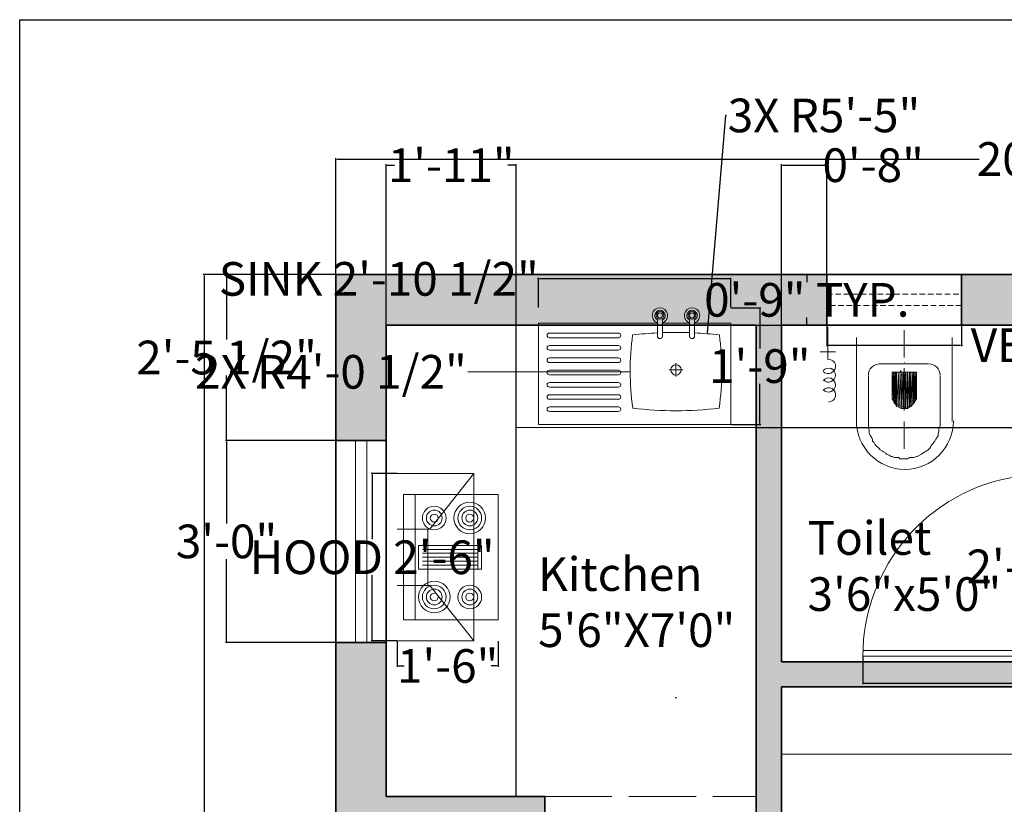
# Model space of a CAD drawing. Units: inches. Extents: x 335 to 688, y 1043 to 1486.
# Tile 4 of 7: x 335 to 510, y 1347 to 1486. Entities that reach past the tile are written whole.
import ezdxf

# ---------------------------------------------------------------- set-up
doc = ezdxf.new("R2010")
doc.units = ezdxf.units.IN
doc.header["$MEASUREMENT"] = 0
doc.linetypes.add('ACAD_ISO02W100', pattern=[15, 12, -3])
doc.linetypes.add('DASHEDX2', pattern=[1.5, 1, -0.5])
for name, color, linetype, lineweight in [('A-ANNO-DIMS', 2, 'Continuous', 18), ('A-ANNO-TTLB', 7, 'Continuous', 25), ('A-AREA-IDEN', 7, 'Continuous', 18), ('A-DOOR', 4, 'Continuous', 18), ('A-EQPM', 8, 'Continuous', 18), ('A-FLOR-CASE', 8, 'Continuous', 18), ('A-FLOR-FIXT', 8, 'Continuous', 18), ('A-GLAZ', 4, 'Continuous', 18), ('A-GLAZ-VENT', 4, 'DASHEDX2', 18), ('A-WALL', 7, 'Continuous', 35), ('A-WALL-OVHD', 7, 'ACAD_ISO02W100', 18), ('A-WALL-PATT', 252, 'Continuous', 13)]:
    doc.layers.add(name, color=color, linetype=linetype, lineweight=lineweight)
doc.styles.get("Standard").update_dxf_attribs({"font": 'arial.ttf'})
doc.dimstyles.get("Standard").update_dxf_attribs({"dimtxt": 6, "dimasz": 0.18, "dimexe": 0.18, "dimexo": 0.0625, "dimgap": 0.09, "dimtad": 0, "dimtih": 1, "dimtoh": 1, "dimdec": 1, "dimzin": 0, "dimdsep": 46, "dimlunit": 3, "dimtxsty": 'Standard', "dimcen": 0.09, "dimadec": 0, "dimazin": 0, "dimtfac": 1, "dimtdec": 1, "dimtofl": 0, "dimtmove": 0, "dimatfit": 3, "dimfxl": 1, "dimtolj": 1, "dimtzin": 0, "dimarcsym": 0})

# ---------------------------------------------------------------- blocks, each defined once
blk = doc.blocks.new('chimmne')
for p, q in [((17.89, 6.07), (-18.11, 6.07)), ((-18.11, 6.07), (-18.11, -10.43)), ((-6.16, -3.43), (-18.11, 6.07)), ((5.94, -3.43), (17.89, 6.07)), ((17.89, 6.07), (17.89, -10.43)), ((-6.16, -3.43), (-6.16, -10.43)), ((5.94, -3.82), (-6.16, -3.82)), ((5.94, -3.43), (5.94, -10.43))]:
    blk.add_line(p, q)
for points in [[(-13.61, -9.12), (-13.61, 11.28), (13.39, 11.28), (13.39, -9.12)], [(-2.66, -5.87), (-2.66, 7.73), (2.44, 7.73), (2.44, -5.87)]]:
    blk.add_lwpolyline(points, close=True)
for points in [[(-2.66, 6.88), (2.44, 6.88)], [(-1.81, 6.88), (-1.81, -5.02)], [(-0.96, -5.02), (-0.96, 6.88)], [(-0.11, 6.88), (-0.11, -5.02)], [(0.74, -5.02), (0.74, 6.88)], [(1.59, 6.88), (1.59, -5.02)], [(13.39, -6.57), (-13.61, -6.57)]]:
    blk.add_lwpolyline(points)
for centre, radius in [((-8.55, 5.18), 3.4), ((-8.55, 5.18), 2.55), ((-8.55, 5.18), 1.7), ((8.44, 5.18), 2.55), ((8.44, 5.18), 1.7), ((-8.55, 5.18), 0.85), ((8.44, 5.18), 0.85), ((-8.55, -2.47), 2.55), ((8.44, -2.47), 3.4), ((8.44, -2.47), 2.55), ((-8.55, -2.47), 1.7), ((-8.55, -2.47), 0.85), ((8.44, -2.47), 1.7), ((8.44, -2.47), 0.85)]:
    blk.add_circle(centre, radius)
blk = doc.blocks.new('A$C799204C7')
for p, q in [((0, 34.2), (17.99, 34.2)), ((0, 0), (0, 34.2)), ((17.99, 13.08), (17.99, 34.2)), ((2.32, 20.01), (2.32, 32.27)), ((3.13, 20.01), (3.13, 32.27)), ((4.48, 20.01), (4.48, 32.27)), ((5.29, 20.01), (5.29, 32.27)), ((6.64, 20.01), (6.64, 32.27)), ((7.45, 20.01), (7.45, 32.27)), ((8.85, 20.01), (8.85, 32.27)), ((9.66, 20.01), (9.66, 32.27)), ((11.01, 20.01), (11.01, 32.27)), ((11.82, 20.01), (11.82, 32.27)), ((13.22, 20.01), (13.22, 32.27)), ((14.03, 20.01), (14.03, 32.27)), ((15.42, 20.01), (15.42, 32.27)), ((16.24, 20.01), (16.24, 32.27)), ((18.59, 13.08), (15.71, 13.08)), ((9.73, 11), (9.73, 8.54)), ((15.71, 12.17), (18.59, 12.17)), ((17.99, 7.36), (17.99, 12.17)), ((8.52, 9.77), (10.9, 9.77)), ((18.59, 7.36), (15.71, 7.36)), ((15.71, 6.45), (18.59, 6.45)), ((17.99, 0), (17.99, 6.45)), ((0, 0), (17.99, 0))]:
    blk.add_line(p, q)
for centre, radius in [((19.38, 12.62), 0.684), ((19.38, 12.62), 0.456), ((9.7, 9.77), 0.916), ((19.38, 6.91), 0.684), ((19.38, 6.91), 0.456)]:
    blk.add_circle(centre, radius)
for centre, radius, start, end in [((2.72, 32.27), 0.407, 0, 180), ((4.88, 32.27), 0.407, 0, 180), ((7.05, 32.27), 0.407, 0, 180), ((9.25, 32.27), 0.407, 0, 180), ((11.42, 32.27), 0.407, 0, 180), ((13.62, 32.27), 0.407, 0, 180), ((15.83, 32.27), 0.407, 0, 180), ((2.72, 20.01), 0.407, 180, 0), ((4.88, 20.01), 0.407, 180, 0), ((7.05, 20.01), 0.407, 180, 0), ((9.25, 20.01), 0.407, 180, 0), ((11.42, 20.01), 0.407, 180, 0), ((13.62, 20.01), 0.407, 180, 0), ((15.83, 20.01), 0.407, 180, 0), ((9.53, -30.19), 48.1, 82.3437, 97.8966), ((67.33, 9.77), 64.88, 173.1952, 186.8048), ((-48.51, 9.77), 64.88, 2.9208, 6.8048), ((15.71, 12.62), 0.456, 90, 270), ((19.38, 12.62), 1.37, 199.6514, 160.3603), ((19.38, 12.62), 0.911, 210.3431, 149.7554), ((-48.51, 9.77), 64.88, 357.8723, 2.115), ((15.71, 6.91), 0.456, 90, 270), ((19.38, 6.91), 1.37, 199.6514, 160.3603), ((19.38, 6.91), 0.911, 210.3431, 149.7554), ((-48.51, 9.77), 64.88, 353.1952, 357.0665), ((9.53, 49.73), 48.1, 262.1034, 277.6563)]:
    blk.add_arc(centre, radius, start, end)
blk = doc.blocks.new('*D3')
at = {"layer": 'A-ANNO-DIMS', "color": 0, "lineweight": -2, "transparency": 16777216}
for p, q in [((391.11, 1441.03), (391.11, 1461.75)), ((391.29, 1461.57), (505.87, 1461.57)), ((630.93, 1461.57), (516.34, 1461.57)), ((631.11, 1441.03), (631.11, 1461.75))]:
    blk.add_line(p, q, dxfattribs=at)
at = {"layer": 'A-ANNO-DIMS', "color": 0, "transparency": 16777216}
for points in [[(391.29, 1461.6), (391.29, 1461.54), (391.11, 1461.57)], [(630.93, 1461.6), (630.93, 1461.54), (631.11, 1461.57)]]:
    blk.add_solid(points, dxfattribs=at)
at = {"layer": 'Defpoints', "color": 0, "transparency": 16777216}
for p in [(631.11, 1461.57), (391.11, 1440.97), (631.11, 1440.97)]:
    blk.add_point(p, dxfattribs=at)
at = {"layer": 'A-ANNO-DIMS', "color": 0, "transparency": 16777216, "insert": (511.11, 1461.57), "char_height": 6, "attachment_point": 5}
blk.add_mtext("\\A1;20'", dxfattribs=at)
blk = doc.blocks.new('*D4')
at = {"layer": 'A-ANNO-DIMS', "color": 0, "lineweight": -2, "transparency": 16777216}
for p, q in [((391.04, 1440.97), (367.42, 1440.97)), ((367.6, 1440.79), (367.6, 1264.12)), ((367.6, 1081.15), (367.6, 1257.81)), ((391.04, 1080.97), (367.42, 1080.97))]:
    blk.add_line(p, q, dxfattribs=at)
at = {"layer": 'A-ANNO-DIMS', "color": 0, "transparency": 16777216}
for points in [[(367.57, 1440.79), (367.63, 1440.79), (367.6, 1440.97)], [(367.57, 1081.15), (367.63, 1081.15), (367.6, 1080.97)]]:
    blk.add_solid(points, dxfattribs=at)
at = {"layer": 'Defpoints', "color": 0, "transparency": 16777216}
for p in [(391.11, 1440.97), (367.6, 1080.97), (391.11, 1080.97)]:
    blk.add_point(p, dxfattribs=at)
at = {"layer": 'A-ANNO-DIMS', "color": 0, "transparency": 16777216, "insert": (367.6, 1260.97), "char_height": 6, "attachment_point": 5}
blk.add_mtext("\\A1;30'", dxfattribs=at)
blk = doc.blocks.new('WC')
h = blk.add_hatch(color=256)
h.paths.add_polyline_path([(17.3, 10.54), (11.83, 10.54), (17.3, 10.32)])
h.paths.add_polyline_path([(11.83, 10.54), (17.3, 10.32), (11.61, 10.32)])
h = blk.add_hatch(color=256)
h.paths.add_polyline_path([(17.3, 10.7), (12.21, 10.7), (17.3, 10.54)])
h.paths.add_polyline_path([(12.21, 10.7), (17.3, 10.54), (11.83, 10.54)])
h = blk.add_hatch(color=256)
h.paths.add_polyline_path([(17.3, 10.92), (12.59, 10.92), (17.3, 10.7)])
h.paths.add_polyline_path([(12.59, 10.92), (17.3, 10.7), (12.21, 10.7)])
h = blk.add_hatch(color=256)
h.paths.add_polyline_path([(17.3, 9.71), (11.08, 9.71), (17.3, 9.33)])
h.paths.add_polyline_path([(11.08, 9.71), (17.3, 9.33), (10.85, 9.33)])
h = blk.add_hatch(color=256)
h.paths.add_polyline_path([(17.3, 9.33), (10.85, 9.33), (17.3, 8.95)])
h.paths.add_polyline_path([(10.85, 9.33), (17.3, 8.95), (10.85, 8.95)])
h = blk.add_hatch(color=256)
h.paths.add_polyline_path([(17.3, 8.95), (10.85, 8.95), (17.3, 8.57)])
h.paths.add_polyline_path([(10.85, 8.95), (17.3, 8.57), (10.85, 8.57)])
h = blk.add_hatch(color=256)
h.paths.add_polyline_path([(17.3, 10.16), (11.23, 10.16), (17.3, 9.71)])
h.paths.add_polyline_path([(11.23, 10.16), (17.3, 9.71), (11.08, 9.71)])
h = blk.add_hatch(color=256)
h.paths.add_polyline_path([(17.3, 10.32), (11.61, 10.32), (17.3, 10.16)])
h.paths.add_polyline_path([(11.61, 10.32), (17.3, 10.16), (11.23, 10.16)])
h = blk.add_hatch(color=256)
h.paths.add_polyline_path([(17.3, 8.57), (10.85, 8.57), (17.3, 8.19)])
h.paths.add_polyline_path([(10.85, 8.57), (17.3, 8.19), (10.85, 8.19)])
h = blk.add_hatch(color=256)
h.paths.add_polyline_path([(17.3, 8.19), (10.85, 8.19), (17.3, 7.81)])
h.paths.add_polyline_path([(10.85, 8.19), (17.3, 7.81), (11.08, 7.81)])
h = blk.add_hatch(color=256)
h.paths.add_polyline_path([(17.3, 7.81), (11.08, 7.81), (17.3, 7.59)])
h.paths.add_polyline_path([(11.08, 7.81), (17.3, 7.59), (11.23, 7.59)])
h = blk.add_hatch(color=256)
h.paths.add_polyline_path([(17.3, 7.59), (11.23, 7.59), (17.3, 7.21)])
h.paths.add_polyline_path([(11.23, 7.59), (17.3, 7.21), (11.61, 7.21)])
h = blk.add_hatch(color=256)
h.paths.add_polyline_path([(17.3, 7.21), (11.61, 7.21), (17.3, 7.05)])
h.paths.add_polyline_path([(11.61, 7.21), (17.3, 7.05), (11.83, 7.05)])
h = blk.add_hatch(color=256)
h.paths.add_polyline_path([(17.3, 7.05), (11.83, 7.05), (17.3, 6.83)])
h.paths.add_polyline_path([(11.83, 7.05), (17.3, 6.83), (12.21, 6.83)])
h = blk.add_hatch(color=256)
h.paths.add_polyline_path([(17.3, 6.83), (12.21, 6.83), (17.3, 6.6)])
h.paths.add_polyline_path([(12.21, 6.83), (17.3, 6.6), (12.59, 6.6)])
h.paths.add_polyline_path([(17.3, 6.6), (12.59, 6.6), (12.97, 6.6)])
for points in [[(20.94, 21.04), (20.94, 23.77), (20.94, 23.77)], [(25.41, 22.4), (19.57, 22.4), (19.57, 22.4)], [(23.52, 17.3), (8.5, 17.3), (8.5, 17.3)], [(9.48, 2.35), (8.72, 2.35), (8.12, 2.35), (7.74, 2.35), (7.36, 2.58), (6.98, 2.58), (6.75, 2.58), (6.37, 2.73), (5.99, 2.73), (5.61, 2.96), (5.39, 3.11), (5.01, 3.34), (4.85, 3.49), (4.48, 3.72), (4.25, 3.94), (3.87, 4.1), (3.64, 4.32), (3.49, 4.48), (3.26, 4.85), (3.11, 5.08), (2.88, 5.46), (2.73, 5.69), (2.5, 6.07), (2.28, 6.45), (2.28, 6.6), (2.12, 7.05), (2.12, 7.43), (2.12, 7.81), (1.9, 8.19), (1.9, 8.8), (1.9, 9.56), (2.12, 9.71), (2.12, 10.16), (2.12, 10.54), (2.28, 10.92), (2.28, 11.08), (2.5, 11.45), (2.73, 11.91), (2.88, 12.06), (3.11, 12.44), (3.26, 12.67), (3.49, 13.05), (3.64, 13.2), (3.87, 13.43), (4.25, 13.81), (4.48, 14.03), (4.85, 14.19), (5.01, 14.41), (5.39, 14.41), (5.61, 14.56), (5.99, 14.79), (6.37, 15.02), (6.75, 15.02), (6.98, 15.02), (7.36, 15.17), (7.74, 15.17), (8.12, 15.17), (8.72, 15.17), (9.48, 15.17)], [(16.69, 15.17), (9.48, 15.17), (9.48, 15.17)], [(18.81, 4.48), (18.81, 13.2), (18.81, 13.2)], [(17.3, 10.92), (12.97, 10.92), (12.97, 10.92)], [(17.3, 6.6), (17.3, 10.92), (17.3, 10.92)], [(8.5, 8.8), (3.64, 8.8), (3.64, 8.8)], [(18.05, 8.8), (10.47, 8.8), (10.47, 8.8)], [(16.84, 9.18), (16.92, 9.18), (16.92, 9.18)], [(16.84, 8.8), (16.84, 8.95), (16.84, 9.18)], [(16.84, 8.8), (16.92, 8.72), (16.92, 8.72)], [(16.84, 8.34), (16.84, 8.57), (16.84, 8.8)], [(19.04, 8.8), (19.04, 8.72), (19.04, 8.72)], [(24.81, 8.8), (19.95, 8.8), (19.95, 8.8)], [(16.84, 8.34), (16.92, 8.34), (16.92, 8.34)], [(17.3, 6.6), (12.97, 6.6), (12.97, 6.6)], [(16.69, 2.35), (9.48, 2.35), (9.48, 2.35)], [(23.52, 0.23), (8.5, 0.23), (8.5, 0.23)]]:
    blk.add_lwpolyline(points)
for points in [[(11.83, 10.54), (17.3, 10.32), (11.61, 10.32)], [(12.21, 10.7), (17.3, 10.54), (11.83, 10.54)], [(17.3, 10.54), (11.83, 10.54), (17.3, 10.32)], [(12.59, 10.92), (17.3, 10.7), (12.21, 10.7)], [(17.3, 10.7), (12.21, 10.7), (17.3, 10.54)], [(12.97, 10.92), (17.3, 10.92), (12.59, 10.92)], [(17.3, 10.92), (12.59, 10.92), (17.3, 10.7)], [(17.3, 10.92), (12.97, 10.92)], [(11.08, 9.71), (17.3, 9.33), (10.85, 9.33)], [(17.3, 9.33), (10.85, 9.33), (17.3, 8.95)], [(10.85, 9.33), (17.3, 8.95), (10.85, 8.95)], [(17.3, 8.95), (10.85, 8.95), (17.3, 8.57)], [(10.85, 8.95), (17.3, 8.57), (10.85, 8.57)], [(11.23, 10.16), (17.3, 9.71), (11.08, 9.71)], [(17.3, 9.71), (11.08, 9.71), (17.3, 9.33)], [(11.61, 10.32), (17.3, 10.16), (11.23, 10.16)], [(17.3, 10.16), (11.23, 10.16), (17.3, 9.71)], [(17.3, 10.32), (11.61, 10.32), (17.3, 10.16)], [(17.3, 8.57), (10.85, 8.57), (17.3, 8.19)], [(10.85, 8.57), (17.3, 8.19), (10.85, 8.19)], [(17.3, 8.19), (10.85, 8.19), (17.3, 7.81)], [(10.85, 8.19), (17.3, 7.81), (11.08, 7.81)], [(17.3, 7.81), (11.08, 7.81), (17.3, 7.59)], [(11.08, 7.81), (17.3, 7.59), (11.23, 7.59)], [(17.3, 7.59), (11.23, 7.59), (17.3, 7.21)], [(11.23, 7.59), (17.3, 7.21), (11.61, 7.21)], [(17.3, 7.21), (11.61, 7.21), (17.3, 7.05)], [(11.61, 7.21), (17.3, 7.05), (11.83, 7.05)], [(17.3, 7.05), (11.83, 7.05), (17.3, 6.83)], [(11.83, 7.05), (17.3, 6.83), (12.21, 6.83)], [(17.3, 6.83), (12.21, 6.83), (17.3, 6.6)], [(12.21, 6.83), (17.3, 6.6), (12.59, 6.6)], [(17.3, 6.6), (12.59, 6.6), (12.97, 6.6)], [(12.59, 6.6), (17.3, 6.6), (17.3, 6.6)]]:
    blk.add_lwpolyline(points, close=True)
for points, knots in [([(11.99, 22.25), (11.99, 21.72), (12.44, 21.19), (12.97, 21.04), (12.97, 21.04), (13.5, 20.88), (14.11, 21.19), (14.41, 21.64), (14.41, 21.64), (14.64, 22.17), (14.56, 22.78), (14.19, 23.16)], [0, 0, 0, 0, 0.083333, 0.083333, 0.083333, 0.083334, 0.166667, 0.166667, 0.166667, 0.166668, 1, 1, 1, 1]), ([(14.19, 23.23), (13.81, 22.86), (13.65, 22.32), (13.88, 21.79), (13.88, 21.79), (14.03, 21.34), (14.49, 21.04), (15.02, 21.04), (15.02, 21.04), (15.55, 21.04), (16.01, 21.34), (16.23, 21.79), (16.23, 21.79), (16.39, 22.32), (16.23, 22.86), (15.85, 23.23)], [0, 0, 0, 0, 0.0625, 0.0625, 0.0625, 0.062501, 0.125, 0.125, 0.125, 0.125001, 0.1875, 0.1875, 0.1875, 0.187501, 1, 1, 1, 1]), ([(15.93, 23.16), (15.55, 22.86), (15.4, 22.25), (15.63, 21.79), (15.63, 21.79), (15.78, 21.34), (16.31, 21.04), (16.76, 21.04), (16.76, 21.04), (17.3, 21.04), (17.75, 21.34), (17.98, 21.79), (17.98, 21.79), (18.13, 22.32), (17.98, 22.86), (17.6, 23.23)], [0, 0, 0, 0, 0.0625, 0.0625, 0.0625, 0.062501, 0.125, 0.125, 0.125, 0.125001, 0.1875, 0.1875, 0.1875, 0.187501, 1, 1, 1, 1]), ([(17.45, 23.23), (17.07, 22.86), (16.92, 22.17), (17.22, 21.72), (17.22, 21.72), (17.52, 21.19), (18.05, 20.88), (18.66, 21.04), (18.66, 21.04), (19.19, 21.19), (19.57, 21.72), (19.57, 22.25)], [0, 0, 0, 0, 0.083333, 0.083333, 0.083333, 0.083334, 0.166667, 0.166667, 0.166667, 0.166668, 1, 1, 1, 1]), ([(8.65, 17.3), (3.87, 17.3), (0, 13.43), (0, 8.65), (0, 8.65), (0, 3.87), (3.87, 0), (8.65, 0)], [0, 0, 0, 0, 0.125, 0.125, 0.125, 0.125001, 1, 1, 1, 1]), ([(13.12, 10.7), (11.99, 10.7), (11.08, 9.79), (11.08, 8.65), (11.08, 8.65), (11.08, 7.51), (11.99, 6.6), (13.12, 6.6)], [0, 0, 0, 0, 0.125, 0.125, 0.125, 0.125001, 1, 1, 1, 1])]:
    blk.add_open_spline(points, degree=3, knots=knots)
for points in [[(18.81, 13.12), (18.81, 14.26), (17.9, 15.17), (16.76, 15.17)], [(16.76, 2.35), (17.9, 2.35), (18.81, 3.26), (18.81, 4.4)]]:
    blk.add_open_spline(points, degree=3)
blk = doc.blocks.new('VENT-24IN')
for p, q in [((0, 0), (0, 24)), ((3.5, 0), (3.5, 24)), ((5.5, 24), (5.5, 0)), ((9, 24), (9, 0))]:
    blk.add_line(p, q)
blk = doc.blocks.new('DOOR-32IN')
for p, q in [((0, 1), (32, 1)), ((32, 0), (32, 1)), ((32, 0), (0, 0)), ((0, 0), (32, 0))]:
    blk.add_line(p, q)
blk.add_arc((32.37, 0), 32.37, 98.6501, 180)
blk = doc.blocks.new('*D27')
at = {"layer": 'A-ANNO-DIMS', "color": 0, "lineweight": -2, "transparency": 16777216}
for p, q in [((478.71, 1431.9), (478.71, 1428.19)), ((502.71, 1431.9), (502.71, 1428.19)), ((478.89, 1428.37), (502.53, 1428.37)), ((502.71, 1428.37), (502.89, 1428.37))]:
    blk.add_line(p, q, dxfattribs=at)
at = {"layer": 'A-ANNO-DIMS', "color": 0, "transparency": 16777216}
for points in [[(478.89, 1428.4), (478.89, 1428.34), (478.71, 1428.37)], [(502.53, 1428.4), (502.53, 1428.34), (502.71, 1428.37)]]:
    blk.add_solid(points, dxfattribs=at)
at = {"layer": 'Defpoints', "color": 0, "transparency": 16777216}
for p in [(478.71, 1431.97), (502.71, 1431.97), (502.71, 1428.37)]:
    blk.add_point(p, dxfattribs=at)
at = {"layer": 'A-ANNO-DIMS', "color": 0, "transparency": 16777216, "insert": (533.76, 1428.37), "char_height": 6, "attachment_point": 5}
blk.add_mtext('\\A1;VENT 2\'-0" TYP.', dxfattribs=at)
blk = doc.blocks.new('*D28')
at = {"layer": 'A-ANNO-DIMS', "color": 0, "lineweight": -2, "transparency": 16777216}
for p, q in [((478.65, 1440.97), (474.93, 1440.97)), ((475.11, 1440.79), (475.11, 1439.62)), ((475.11, 1432.15), (475.11, 1433.31)), ((478.65, 1431.97), (474.93, 1431.97))]:
    blk.add_line(p, q, dxfattribs=at)
at = {"layer": 'A-ANNO-DIMS', "color": 0, "transparency": 16777216}
for points in [[(475.08, 1440.79), (475.14, 1440.79), (475.11, 1440.97)], [(475.08, 1432.15), (475.14, 1432.15), (475.11, 1431.97)]]:
    blk.add_solid(points, dxfattribs=at)
at = {"layer": 'Defpoints', "color": 0, "transparency": 16777216}
for p in [(478.71, 1440.97), (475.11, 1431.97), (478.71, 1431.97)]:
    blk.add_point(p, dxfattribs=at)
at = {"layer": 'A-ANNO-DIMS', "color": 0, "transparency": 16777216, "insert": (475.11, 1436.47), "char_height": 6, "attachment_point": 5}
blk.add_mtext('\\A1;0\'-9" TYP.', dxfattribs=at)
blk = doc.blocks.new('*D29')
at = {"layer": 'A-ANNO-DIMS', "color": 0, "lineweight": -2, "transparency": 16777216}
for p, q in [((485.11, 1372.9), (485.11, 1367.99)), ((517.11, 1372.9), (517.11, 1367.99)), ((485.29, 1368.17), (516.93, 1368.17)), ((517.11, 1368.17), (517.29, 1368.17))]:
    blk.add_line(p, q, dxfattribs=at)
at = {"layer": 'A-ANNO-DIMS', "color": 0, "transparency": 16777216}
for points in [[(485.29, 1368.2), (485.29, 1368.14), (485.11, 1368.17)], [(516.93, 1368.2), (516.93, 1368.14), (517.11, 1368.17)]]:
    blk.add_solid(points, dxfattribs=at)
at = {"layer": 'Defpoints', "color": 0, "transparency": 16777216}
for p in [(485.11, 1372.97), (517.11, 1372.97), (517.11, 1368.17)]:
    blk.add_point(p, dxfattribs=at)
at = {"layer": 'A-ANNO-DIMS', "color": 0, "transparency": 16777216, "insert": (557.67, 1368.17), "char_height": 6, "attachment_point": 5}
blk.add_mtext('\\A1;WC DOOR 2\'-8" TYP.', dxfattribs=at)
blk = doc.blocks.new('*D30')
at = {"layer": 'A-ANNO-DIMS', "color": 0, "lineweight": -2, "transparency": 16777216}
for p, q in [((517.17, 1404.97), (522.09, 1404.97)), ((521.91, 1404.79), (521.91, 1392.12)), ((521.91, 1373.15), (521.91, 1385.81)), ((517.17, 1372.97), (522.09, 1372.97))]:
    blk.add_line(p, q, dxfattribs=at)
at = {"layer": 'A-ANNO-DIMS', "color": 0, "transparency": 16777216}
for points in [[(521.88, 1404.79), (521.94, 1404.79), (521.91, 1404.97)], [(521.88, 1373.15), (521.94, 1373.15), (521.91, 1372.97)]]:
    blk.add_solid(points, dxfattribs=at)
at = {"layer": 'Defpoints', "color": 0, "transparency": 16777216}
for p in [(517.11, 1404.97), (521.91, 1404.97), (517.11, 1372.97)]:
    blk.add_point(p, dxfattribs=at)
at = {"layer": 'A-ANNO-DIMS', "color": 0, "transparency": 16777216, "insert": (521.91, 1388.97), "char_height": 6, "attachment_point": 5}
blk.add_mtext('\\A1;2\'-8" TYP.', dxfattribs=at)
blk = doc.blocks.new('*D35')
at = {"layer": 'A-ANNO-DIMS', "color": 0, "lineweight": -2, "transparency": 16777216}
for p, q in [((402.01, 1405.5), (397.42, 1405.5)), ((397.6, 1405.32), (397.6, 1393.79)), ((397.6, 1375.87), (397.6, 1387.4)), ((402.01, 1375.69), (397.42, 1375.69))]:
    blk.add_line(p, q, dxfattribs=at)
at = {"layer": 'A-ANNO-DIMS', "color": 0, "transparency": 16777216}
for points in [[(397.57, 1405.32), (397.63, 1405.32), (397.6, 1405.5)], [(397.57, 1375.87), (397.63, 1375.87), (397.6, 1375.69)]]:
    blk.add_solid(points, dxfattribs=at)
at = {"layer": 'Defpoints', "color": 0, "transparency": 16777216}
for p in [(402.07, 1405.5), (397.6, 1375.69), (402.07, 1375.69)]:
    blk.add_point(p, dxfattribs=at)
at = {"layer": 'A-ANNO-DIMS', "color": 0, "transparency": 16777216, "insert": (397.6, 1390.59), "char_height": 6, "attachment_point": 5}
blk.add_mtext('\\A1;HOOD 2\'-6"', dxfattribs=at)
blk = doc.blocks.new('*D36')
at = {"layer": 'A-ANNO-DIMS', "color": 0, "lineweight": -2, "transparency": 16777216}
for p, q in [((402.07, 1375.63), (402.07, 1371.04)), ((420.05, 1375.63), (420.05, 1371.04)), ((402.25, 1371.22), (403.28, 1371.22)), ((419.87, 1371.22), (418.84, 1371.22))]:
    blk.add_line(p, q, dxfattribs=at)
at = {"layer": 'A-ANNO-DIMS', "color": 0, "transparency": 16777216}
for points in [[(402.25, 1371.25), (402.25, 1371.19), (402.07, 1371.22)], [(419.87, 1371.25), (419.87, 1371.19), (420.05, 1371.22)]]:
    blk.add_solid(points, dxfattribs=at)
at = {"layer": 'Defpoints', "color": 0, "transparency": 16777216}
for p in [(402.07, 1375.69), (420.05, 1375.69), (420.05, 1371.22)]:
    blk.add_point(p, dxfattribs=at)
at = {"layer": 'A-ANNO-DIMS', "color": 0, "transparency": 16777216, "insert": (411.06, 1371.22), "char_height": 6, "attachment_point": 5}
blk.add_mtext('\\A1;1\'-6"', dxfattribs=at)
blk = doc.blocks.new('*D37')
at = {"layer": 'A-ANNO-DIMS', "color": 0, "lineweight": -2, "transparency": 16777216}
for p, q in [((427.27, 1440.21), (427.09, 1440.21)), ((427.27, 1435.12), (427.27, 1440.39)), ((461.4, 1440.21), (427.45, 1440.21)), ((461.58, 1435.12), (461.58, 1440.39))]:
    blk.add_line(p, q, dxfattribs=at)
at = {"layer": 'A-ANNO-DIMS', "color": 0, "transparency": 16777216}
for points in [[(427.45, 1440.24), (427.45, 1440.18), (427.27, 1440.21)], [(461.4, 1440.24), (461.4, 1440.18), (461.58, 1440.21)]]:
    blk.add_solid(points, dxfattribs=at)
at = {"layer": 'Defpoints', "color": 0, "transparency": 16777216}
for p in [(427.27, 1440.21), (427.27, 1435.06), (461.58, 1435.06)]:
    blk.add_point(p, dxfattribs=at)
at = {"layer": 'A-ANNO-DIMS', "color": 0, "transparency": 16777216, "insert": (398.77, 1440.21), "char_height": 6, "attachment_point": 5}
blk.add_mtext('\\A1;SINK 2\'-10 1/2"', dxfattribs=at)
blk = doc.blocks.new('*D38')
at = {"layer": 'A-ANNO-DIMS', "color": 0, "lineweight": -2, "transparency": 16777216}
for p, q in [((461.64, 1435.06), (466.91, 1435.06)), ((466.73, 1434.88), (466.73, 1427.81)), ((466.73, 1414.43), (466.73, 1421.5)), ((461.64, 1414.25), (466.91, 1414.25))]:
    blk.add_line(p, q, dxfattribs=at)
at = {"layer": 'A-ANNO-DIMS', "color": 0, "transparency": 16777216}
for points in [[(466.7, 1434.88), (466.76, 1434.88), (466.73, 1435.06)], [(466.7, 1414.43), (466.76, 1414.43), (466.73, 1414.25)]]:
    blk.add_solid(points, dxfattribs=at)
at = {"layer": 'Defpoints', "color": 0, "transparency": 16777216}
for p in [(461.58, 1435.06), (466.73, 1435.06), (461.58, 1414.25)]:
    blk.add_point(p, dxfattribs=at)
at = {"layer": 'A-ANNO-DIMS', "color": 0, "transparency": 16777216, "insert": (466.73, 1424.66), "char_height": 6, "attachment_point": 5}
blk.add_mtext('\\A1;1\'-9"', dxfattribs=at)
blk = doc.blocks.new('*D47')
at = {"layer": 'A-ANNO-DIMS', "color": 0, "lineweight": -2, "transparency": 16777216}
for p, q in [((391.04, 1411.42), (371.43, 1411.42)), ((371.61, 1411.24), (371.61, 1396.58)), ((371.61, 1375.6), (371.61, 1390.27)), ((391.04, 1375.42), (371.43, 1375.42))]:
    blk.add_line(p, q, dxfattribs=at)
at = {"layer": 'A-ANNO-DIMS', "color": 0, "transparency": 16777216}
for points in [[(371.58, 1411.24), (371.64, 1411.24), (371.61, 1411.42)], [(371.58, 1375.6), (371.64, 1375.6), (371.61, 1375.42)]]:
    blk.add_solid(points, dxfattribs=at)
at = {"layer": 'Defpoints', "color": 0, "transparency": 16777216}
for p in [(371.61, 1411.42), (391.11, 1411.42), (391.11, 1375.42)]:
    blk.add_point(p, dxfattribs=at)
at = {"layer": 'A-ANNO-DIMS', "color": 0, "transparency": 16777216, "insert": (371.61, 1393.42), "char_height": 6, "attachment_point": 5}
blk.add_mtext('\\A1;3\'-0"', dxfattribs=at)
blk = doc.blocks.new('*D50')
at = {"layer": 'A-ANNO-DIMS', "color": 0, "lineweight": -2, "transparency": 16777216}
for p, q in [((391.04, 1440.97), (371.43, 1440.97)), ((371.61, 1440.79), (371.61, 1429.39)), ((371.61, 1411.6), (371.61, 1423)), ((391.04, 1411.42), (371.43, 1411.42))]:
    blk.add_line(p, q, dxfattribs=at)
at = {"layer": 'A-ANNO-DIMS', "color": 0, "transparency": 16777216}
for points in [[(371.58, 1440.79), (371.64, 1440.79), (371.61, 1440.97)], [(371.58, 1411.6), (371.64, 1411.6), (371.61, 1411.42)]]:
    blk.add_solid(points, dxfattribs=at)
at = {"layer": 'Defpoints', "color": 0, "transparency": 16777216}
for p in [(371.61, 1440.97), (391.11, 1440.97), (391.11, 1411.42)]:
    blk.add_point(p, dxfattribs=at)
at = {"layer": 'A-ANNO-DIMS', "color": 0, "transparency": 16777216, "insert": (371.61, 1426.19), "char_height": 6, "attachment_point": 5}
blk.add_mtext('\\A1;2\'-5 1/2"', dxfattribs=at)
blk = doc.blocks.new('*D54')
at = {"layer": 'A-ANNO-DIMS', "color": 0, "lineweight": -2, "transparency": 16777216}
for p, q in [((470.61, 1432.03), (470.61, 1460.65)), ((470.79, 1460.47), (478.53, 1460.47)), ((478.71, 1432.03), (478.71, 1460.65)), ((478.71, 1460.47), (478.89, 1460.47))]:
    blk.add_line(p, q, dxfattribs=at)
at = {"layer": 'A-ANNO-DIMS', "color": 0, "transparency": 16777216}
for points in [[(470.79, 1460.5), (470.79, 1460.44), (470.61, 1460.47)], [(478.53, 1460.5), (478.53, 1460.44), (478.71, 1460.47)]]:
    blk.add_solid(points, dxfattribs=at)
at = {"layer": 'Defpoints', "color": 0, "transparency": 16777216}
for p in [(478.71, 1460.47), (470.61, 1431.97), (478.71, 1431.97)]:
    blk.add_point(p, dxfattribs=at)
at = {"layer": 'A-ANNO-DIMS', "color": 0, "transparency": 16777216, "insert": (486.95, 1460.47), "char_height": 6, "attachment_point": 5}
blk.add_mtext('\\A1;0\'-8"', dxfattribs=at)
blk = doc.blocks.new('*D61')
at = {"layer": 'A-ANNO-DIMS', "color": 0, "lineweight": -2, "transparency": 16777216}
for p, q in [((428.36, 1347.9), (428.36, 1061.29)), ((466.11, 1347.9), (466.11, 1061.29)), ((428.54, 1061.47), (432.18, 1061.47)), ((465.93, 1061.47), (462.29, 1061.47))]:
    blk.add_line(p, q, dxfattribs=at)
at = {"layer": 'A-ANNO-DIMS', "color": 0, "transparency": 16777216}
for points in [[(428.54, 1061.5), (428.54, 1061.44), (428.36, 1061.47)], [(465.93, 1061.5), (465.93, 1061.44), (466.11, 1061.47)]]:
    blk.add_solid(points, dxfattribs=at)
at = {"layer": 'Defpoints', "color": 0, "transparency": 16777216}
for p in [(428.36, 1347.97), (466.11, 1347.97), (466.11, 1061.47)]:
    blk.add_point(p, dxfattribs=at)
at = {"layer": 'A-ANNO-DIMS', "color": 0, "transparency": 16777216, "insert": (447.24, 1061.47), "char_height": 6, "attachment_point": 5}
blk.add_mtext('\\A1;3\'-1 1/2"', dxfattribs=at)
blk = doc.blocks.new('*D62')
at = {"layer": 'A-ANNO-DIMS', "color": 0, "lineweight": -2, "transparency": 16777216}
for p, q in [((400.11, 1348.03), (400.11, 1460.65)), ((400.29, 1460.47), (401.58, 1460.47)), ((423.1, 1460.47), (421.81, 1460.47)), ((423.28, 1348.03), (423.28, 1460.65))]:
    blk.add_line(p, q, dxfattribs=at)
at = {"layer": 'A-ANNO-DIMS', "color": 0, "transparency": 16777216}
for points in [[(400.29, 1460.5), (400.29, 1460.44), (400.11, 1460.47)], [(423.1, 1460.5), (423.1, 1460.44), (423.28, 1460.47)]]:
    blk.add_solid(points, dxfattribs=at)
at = {"layer": 'Defpoints', "color": 0, "transparency": 16777216}
for p in [(423.28, 1460.47), (400.11, 1347.97), (423.28, 1347.97)]:
    blk.add_point(p, dxfattribs=at)
at = {"layer": 'A-ANNO-DIMS', "color": 0, "transparency": 16777216, "insert": (411.69, 1460.47), "char_height": 6, "attachment_point": 5}
blk.add_mtext('\\A1;1\'-11"', dxfattribs=at)
blk = doc.blocks.new('*D63')
at = {"layer": 'A-ANNO-DIMS', "color": 0, "lineweight": -2, "transparency": 16777216}
for p, q in [((466.17, 1431.97), (650.79, 1431.97)), ((650.61, 1431.79), (650.61, 1426.01)), ((650.61, 1413.92), (650.61, 1419.7)), ((466.17, 1413.74), (650.79, 1413.74))]:
    blk.add_line(p, q, dxfattribs=at)
at = {"layer": 'A-ANNO-DIMS', "color": 0, "transparency": 16777216}
for points in [[(650.58, 1431.79), (650.64, 1431.79), (650.61, 1431.97)], [(650.58, 1413.92), (650.64, 1413.92), (650.61, 1413.74)]]:
    blk.add_solid(points, dxfattribs=at)
at = {"layer": 'Defpoints', "color": 0, "transparency": 16777216}
for p in [(466.11, 1431.97), (650.61, 1431.97), (466.11, 1413.74)]:
    blk.add_point(p, dxfattribs=at)
at = {"layer": 'A-ANNO-DIMS', "color": 0, "transparency": 16777216, "insert": (650.61, 1422.85), "char_height": 6, "attachment_point": 5}
blk.add_mtext('\\A1;1\'-6"', dxfattribs=at)
blk = doc.blocks.new('*D69')
at = {"layer": 'A-ANNO-DIMS', "color": 0, "lineweight": -2, "transparency": 16777216}
for p, q in [((460.62, 1469.34), (457.32, 1430.61)), ((460.8, 1469.34), (460.62, 1469.34)), ((451.69, 1365.58), (451.87, 1365.58)), ((451.78, 1365.49), (451.78, 1365.67))]:
    blk.add_line(p, q, dxfattribs=at)
at = {"layer": 'A-ANNO-DIMS', "color": 0, "transparency": 16777216}
blk.add_solid([(457.29, 1430.61), (457.35, 1430.61), (457.3, 1430.43)], dxfattribs=at)
at = {"layer": 'Defpoints', "color": 0, "transparency": 16777216}
for p in [(457.3, 1430.43), (451.78, 1365.58)]:
    blk.add_point(p, dxfattribs=at)
at = {"layer": 'A-ANNO-DIMS', "color": 0, "transparency": 16777216, "insert": (478.18, 1469.34), "char_height": 6, "attachment_point": 5}
blk.add_mtext('\\A1;3X R5\'-5"', dxfattribs=at)
blk = doc.blocks.new('*D70')
at = {"layer": 'A-ANNO-DIMS', "color": 0, "lineweight": -2, "transparency": 16777216}
for p, q in [((414.66, 1423.64), (443.43, 1423.7)), ((491.77, 1423.8), (491.95, 1423.8)), ((491.86, 1423.71), (491.86, 1423.89))]:
    blk.add_line(p, q, dxfattribs=at)
at = {"layer": 'A-ANNO-DIMS', "color": 0, "transparency": 16777216}
blk.add_solid([(443.43, 1423.73), (443.43, 1423.67), (443.61, 1423.7)], dxfattribs=at)
at = {"layer": 'Defpoints', "color": 0, "transparency": 16777216}
for p in [(443.61, 1423.7), (491.86, 1423.8)]:
    blk.add_point(p, dxfattribs=at)
at = {"layer": 'A-ANNO-DIMS', "color": 0, "transparency": 16777216, "insert": (390.23, 1423.64), "char_height": 6, "attachment_point": 5}
blk.add_mtext('\\A1;2X R4\'-0 1/2"', dxfattribs=at)

msp = doc.modelspace()

# ---------------------------------------------------------------- hatches: boundary and pattern name
at = {"layer": 'A-WALL-PATT'}
h = msp.add_hatch(color=256, dxfattribs=at)
h.dxf.hatch_style = 1
h.paths.add_polyline_path([(478.71, 1440.97), (391.11, 1440.97), (391.11, 1411.42), (400.11, 1411.42), (400.11, 1431.97), (466.11, 1431.97), (466.11, 1347.97), (466.11, 1343.47), (470.61, 1343.47), (470.61, 1367.47), (512.61, 1367.47), (512.61, 1350.97), (517.11, 1350.97), (517.11, 1372.97), (512.61, 1372.97), (512.61, 1371.97), (470.61, 1371.97), (470.61, 1431.97), (478.71, 1431.97)])
h.paths.add_polyline_path([(631.11, 1440.97), (502.71, 1440.97), (502.71, 1431.97), (512.61, 1431.97), (512.61, 1404.97), (517.11, 1404.97), (517.11, 1431.97), (622.11, 1431.97), (622.11, 1401.6), (631.11, 1401.6)])
h.paths.add_polyline_path([(631.11, 1341.6), (622.11, 1341.6), (622.11, 1313.47), (517.11, 1313.47), (517.11, 1314.47), (512.61, 1314.47), (512.61, 1313.47), (512.61, 1307.97), (517.11, 1307.97), (517.11, 1308.97), (553.11, 1308.97), (553.11, 1262.47), (558.61, 1262.47), (558.61, 1266.97), (557.61, 1266.97), (557.61, 1308.97), (622.11, 1308.97), (622.11, 1297.63), (631.11, 1297.63)])
h.paths.add_polyline_path([(631.11, 1273.63), (622.11, 1273.63), (622.11, 1266.97), (590.61, 1266.97), (590.61, 1262.47), (622.11, 1262.47), (622.11, 1230.86), (631.11, 1230.86)])
h.paths.add_polyline_path([(400.11, 1253.85), (391.11, 1253.85), (391.11, 1132.26), (400.11, 1132.26), (400.11, 1149.97), (411.11, 1149.97), (411.11, 1154.47), (400.11, 1154.47)], flags=17)
h.paths.add_polyline_path([(400.11, 1375.42), (391.11, 1375.42), (391.11, 1313.85), (400.11, 1313.85), (400.11, 1343.47), (428.36, 1343.47), (428.36, 1347.97), (400.11, 1347.97)])

# ---------------------------------------------------------------- linework, layer by layer
at = {"layer": 'A-ANNO-TTLB'}
msp.add_lwpolyline([(334.72, 1486.4), (681.01, 1486.4), (681.01, 1043.03), (334.72, 1043.03)], close=True, dxfattribs=at)
at = {"layer": 'A-FLOR-CASE'}
for p, q in [((423.28, 1347.97), (423.28, 1413.74)), ((423.28, 1413.74), (466.11, 1413.74)), ((470.61, 1355.47), (470.61, 1355.47)), ((470.61, 1355.47), (512.61, 1355.47))]:
    msp.add_line(p, q, dxfattribs=at)
at = {"layer": 'A-GLAZ'}
for p, q in [((391.11, 1375.42), (391.11, 1411.42)), ((394.61, 1375.42), (394.61, 1411.42)), ((396.61, 1411.42), (396.61, 1375.42)), ((400.11, 1411.42), (400.11, 1375.42))]:
    msp.add_line(p, q, dxfattribs=at)
at = {"layer": 'A-WALL'}
for p, q in [((391.11, 1440.97), (631.11, 1440.97)), ((391.11, 1440.97), (391.11, 1080.97)), ((478.71, 1440.97), (478.71, 1431.97)), ((502.71, 1431.97), (502.71, 1440.97)), ((400.11, 1431.97), (400.11, 1347.97)), ((400.11, 1431.97), (466.11, 1431.97)), ((466.11, 1431.97), (466.11, 1347.97)), ((470.61, 1431.97), (470.61, 1371.97)), ((470.61, 1431.97), (512.61, 1431.97)), ((391.11, 1411.42), (400.11, 1411.42)), ((400.11, 1375.42), (391.11, 1375.42)), ((470.61, 1371.97), (512.61, 1371.97)), ((470.61, 1367.47), (512.61, 1367.47)), ((470.61, 1367.47), (470.61, 1343.47)), ((400.11, 1347.97), (428.36, 1347.97)), ((428.36, 1347.97), (428.36, 1343.47)), ((466.11, 1347.97), (466.11, 1343.47))]:
    msp.add_line(p, q, dxfattribs=at)
at = {"layer": 'A-WALL-OVHD'}
msp.add_line((428.36, 1347.97), (466.11, 1347.97), dxfattribs=at)

# ---------------------------------------------------------------- block references
at = {"layer": 'A-DOOR'}
msp.add_blockref('DOOR-32IN', (485.11, 1372.97), dxfattribs=at)
at = {"layer": 'A-EQPM', "xscale": 0.8280321260258986, "yscale": 0.8280321260258986, "zscale": 0.8280321260258986, "rotation": 270}
msp.add_blockref('chimmne', (410.71, 1390.5), dxfattribs=at)
at = {"layer": 'A-FLOR-FIXT', "xscale": 1.0032, "yscale": 1.0032, "zscale": 1.0032, "rotation": 89.99999999999999}
msp.add_blockref('A$C799204C7', (461.58, 1414.25), dxfattribs=at)
at = {"layer": 'A-FLOR-FIXT', "rotation": 90.0000000000282}
msp.add_blockref('WC', (501.26, 1406.26), dxfattribs=at)
at = {"layer": 'A-GLAZ-VENT', "rotation": 269.9999999999995}
msp.add_blockref('VENT-24IN', (478.71, 1440.97), dxfattribs=at)

# ---------------------------------------------------------------- texts
at = {"layer": 'A-AREA-IDEN', "char_height": 6, "attachment_point": 1}
for s, width, insert in [('Toilet\\P3\'6"x5\'0"', 38.8438, (475.25, 1397.03)), ('Kitchen\\P5\'6"X7\'0"', 35.2248, (427.19, 1390.6))]:
    msp.add_mtext_dynamic_manual_height_columns(s, width=width, gutter_width=1, heights=[0], dxfattribs=dict(at, insert=insert))

# ---------------------------------------------------------------- dimensions: what is measured, and where the dimension line sits
at = {"layer": 'A-ANNO-DIMS'}
for center, mpoint, text, picture, middle in [((451.78, 1365.58), (457.3, 1430.43), '3X <>', '*D69', (478.18, 1469.34)), ((491.86, 1423.8), (443.61, 1423.7), '2X <>', '*D70', (414.66, 1423.64))]:
    dim = msp.add_radius_dim(center=center, mpoint=mpoint, text=text, dimstyle='Standard', override={"dimdec": 1, "dimlfac": 1, "dimrnd": 0, "dimzin": 1, "dimdsep": 46, "dimlunit": 4, "dimfrac": 2}, dxfattribs=at)
    dim.commit()
    dim.dimension.update_dxf_attribs({"geometry": picture, "text_midpoint": middle, "dimtype": 164})
for base, p1, p2, override, picture, middle in [((631.11, 1461.57), (391.11, 1440.97), (631.11, 1440.97), {"dimclrd": 0, "dimclre": 0, "dimclrt": 0}, '*D3', (511.11, 1461.57)), ((423.28, 1460.47), (400.11, 1347.97), (423.28, 1347.97), {"dimdec": 1, "dimlfac": 1, "dimrnd": 0, "dimzin": 1, "dimdsep": 46, "dimlunit": 4, "dimfrac": 2}, '*D62', (411.69, 1460.47)), ((478.71, 1460.47), (470.61, 1431.97), (478.71, 1431.97), {"dimdec": 1, "dimlfac": 1, "dimrnd": 0, "dimzin": 1, "dimdsep": 46, "dimlunit": 4, "dimfrac": 2}, '*D54', (486.95, 1460.47)), ((420.05, 1371.22), (402.07, 1375.69), (420.05, 1375.69), {"dimdec": 1, "dimlfac": 1, "dimrnd": 0, "dimzin": 1, "dimdsep": 46, "dimlunit": 4, "dimfrac": 2}, '*D36', (411.06, 1371.22)), ((466.1064, 1061.4667), (428.3646, 1347.9667), (466.1064, 1347.9667), {"dimdec": 1, "dimlfac": 1, "dimrnd": 0, "dimzin": 1, "dimdsep": 46, "dimlunit": 4, "dimfrac": 2}, '*D61', (447.2355, 1061.4667))]:
    dim = msp.add_linear_dim(base=base, p1=p1, p2=p2, dimstyle='Standard', override=override, dxfattribs=at)
    dim.commit()
    dim.dimension.update_dxf_attribs({"geometry": picture, "text_midpoint": middle})
for base, p1, p2, angle, text, picture, middle in [((427.27, 1440.21), (461.58, 1435.06), (427.27, 1435.06), 180, 'SINK <>', '*D37', (398.77, 1440.21)), ((475.11, 1431.97), (478.71, 1440.97), (478.71, 1431.97), 270, '<> TYP.', '*D28', (475.11, 1436.47)), ((397.6, 1375.69), (402.07, 1405.5), (402.07, 1375.69), 270, 'HOOD <>', '*D35', (397.6, 1390.59)), ((521.91, 1404.97), (517.11, 1372.97), (517.11, 1404.97), 90, '<> TYP.', '*D30', (521.91, 1388.97))]:
    dim = msp.add_linear_dim(base=base, p1=p1, p2=p2, angle=angle, text=text, dimstyle='Standard', override={"dimdec": 1, "dimlfac": 1, "dimrnd": 0, "dimzin": 1, "dimdsep": 46, "dimlunit": 4, "dimfrac": 2}, dxfattribs=at)
    dim.commit()
    dim.dimension.update_dxf_attribs({"geometry": picture, "text_midpoint": middle})
for base, p1, p2, text, picture, middle in [((502.71, 1428.37), (478.71, 1431.97), (502.71, 1431.97), 'VENT <> TYP.', '*D27', (533.76, 1428.37)), ((517.11, 1368.17), (485.11, 1372.97), (517.11, 1372.97), 'WC DOOR <> TYP.', '*D29', (557.67, 1368.17))]:
    dim = msp.add_linear_dim(base=base, p1=p1, p2=p2, text=text, dimstyle='Standard', override={"dimdec": 1, "dimlfac": 1, "dimrnd": 0, "dimzin": 1, "dimdsep": 46, "dimlunit": 4, "dimfrac": 2}, dxfattribs=at)
    dim.commit()
    dim.dimension.update_dxf_attribs({"geometry": picture, "text_midpoint": middle})
for base, p1, p2, override, picture, middle in [((371.6064, 1440.9667), (391.1064, 1411.4226), (391.1064, 1440.9667), {"dimdec": 1, "dimlfac": 1, "dimrnd": 0, "dimzin": 1, "dimdsep": 46, "dimlunit": 4, "dimfrac": 2}, '*D50', (371.6064, 1426.1947)), ((367.6, 1080.97), (391.11, 1440.97), (391.11, 1080.97), {"dimclrd": 0, "dimclre": 0, "dimclrt": 0}, '*D4', (367.6, 1260.97)), ((466.73, 1435.06), (461.58, 1414.25), (461.58, 1435.06), {"dimdec": 1, "dimlfac": 1, "dimrnd": 0, "dimzin": 1, "dimdsep": 46, "dimlunit": 4, "dimfrac": 2}, '*D38', (466.73, 1424.66)), ((650.61, 1431.97), (466.11, 1413.74), (466.11, 1431.97), {"dimdec": 1, "dimlfac": 1, "dimrnd": 0, "dimzin": 1, "dimdsep": 46, "dimlunit": 4, "dimfrac": 2}, '*D63', (650.61, 1422.85)), ((371.61, 1411.42), (391.11, 1375.42), (391.11, 1411.42), {"dimdec": 1, "dimlfac": 1, "dimrnd": 0, "dimzin": 1, "dimdsep": 46, "dimlunit": 4, "dimfrac": 2}, '*D47', (371.61, 1393.42))]:
    dim = msp.add_linear_dim(base=base, p1=p1, p2=p2, angle=90, dimstyle='Standard', override=override, dxfattribs=at)
    dim.commit()
    dim.dimension.update_dxf_attribs({"geometry": picture, "text_midpoint": middle})

doc.saveas('drawing.dxf')
